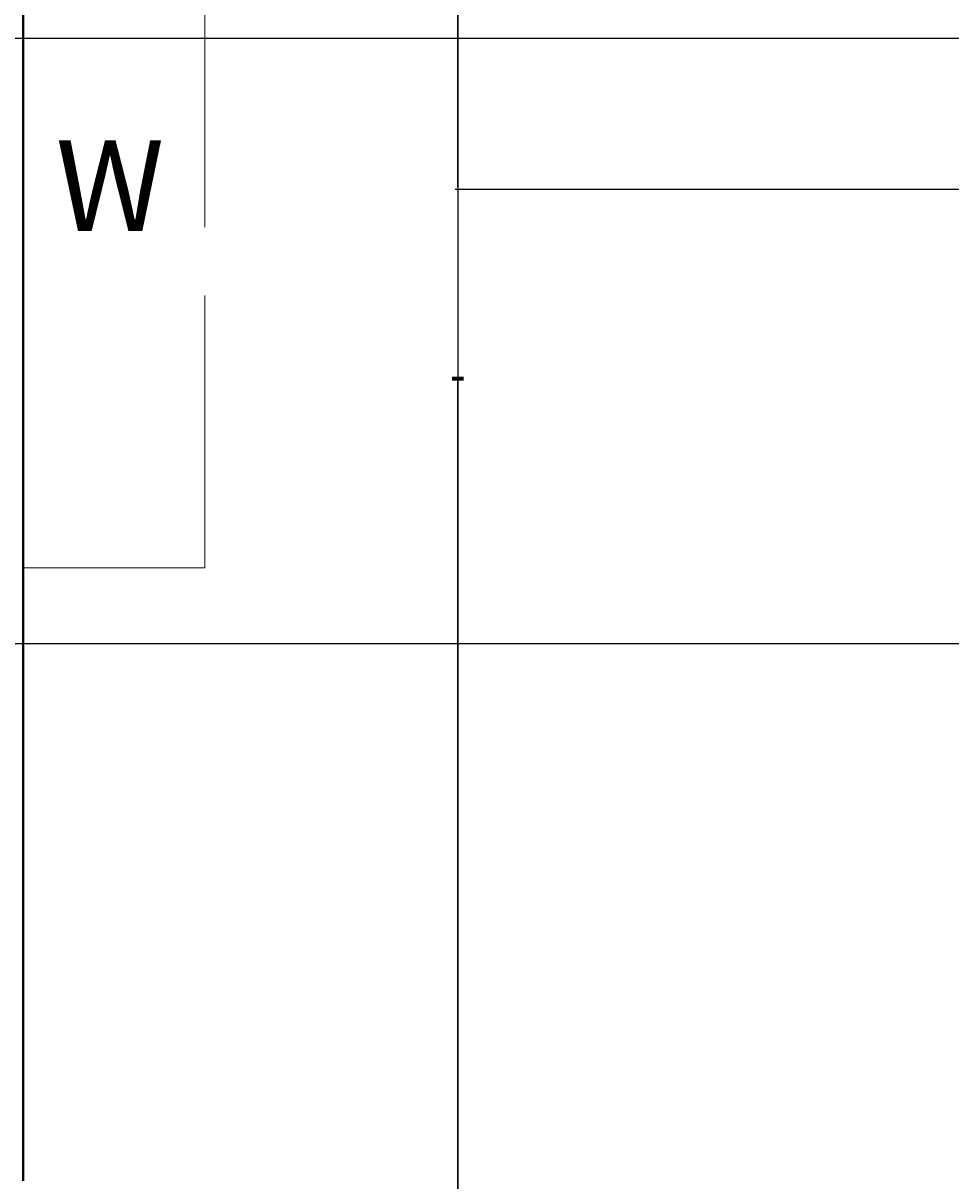
# Model space of a CAD drawing. Units: inches. Extents: x -301 to 715, y -607 to 364.
# Tile 103 of 141: x 133 to 194, y -10 to 67. Entities that reach past the tile are written whole.
import ezdxf

# ---------------------------------------------------------------- set-up
doc = ezdxf.new("R2010")
doc.units = ezdxf.units.IN
doc.header["$MEASUREMENT"] = 0
doc.linetypes.add('ACAD_ISO02W100', pattern=[15, 12, -3])
for name, color, linetype, lineweight in [('A-ANNO-DIMS', 2, 'Continuous', 18), ('A-ANNO-TEXT', 4, 'Continuous', 18), ('A-GLAZ-OVHD', 2, 'ACAD_ISO02W100', 18), ('A-WALL', 3, 'Continuous', 40)]:
    doc.layers.add(name, color=color, linetype=linetype, lineweight=lineweight)
doc.styles.get("Standard").update_dxf_attribs({"font": 'arial.ttf'})
doc.dimstyles.get("Standard").update_dxf_attribs({"dimtxt": 0.18, "dimasz": 0.18, "dimexe": 0.18, "dimexo": 0.0625, "dimgap": 0.09, "dimtad": 0, "dimtih": 1, "dimtoh": 1, "dimdec": 1, "dimzin": 0, "dimdsep": 46, "dimlunit": 4, "dimtxsty": 'Standard', "dimcen": 0.09, "dimclrd": 3, "dimclre": 4, "dimclrt": 6, "dimadec": 0, "dimazin": 0, "dimtfac": 1, "dimtdec": 1, "dimtofl": 0, "dimtmove": 0, "dimatfit": 3, "dimfxl": 1, "dimtfill": 2, "dimtfillclr": 51, "dimtolj": 1, "dimtzin": 0, "dimarcsym": 0})

# ---------------------------------------------------------------- blocks, each defined once
blk = doc.blocks.new('WIN-SHADE-50')
at = {"ltscale": 1.5}
for p, q in [((0, 0), (0, 12)), ((50, 12), (0, 12)), ((50, 0), (50, 12)), ((5, 0), (0, 0)), ((45, 0), (50, 0))]:
    blk.add_line(p, q, dxfattribs=at)
blk = doc.blocks.new('*D149')
at = {"layer": 'A-ANNO-DIMS', "color": 4, "lineweight": -2, "transparency": 16777216}
for p, q in [((-51.541, 65.682), (233.659, 65.682)), ((-51.541, 25.682), (233.659, 25.682))]:
    blk.add_line(p, q, dxfattribs=at)
at = {"layer": 'A-ANNO-DIMS', "color": 3, "lineweight": -2, "transparency": 16777216}
for p, q in [((233.479, 65.502), (233.479, 45.864)), ((233.479, 25.862), (233.479, 45.5))]:
    blk.add_line(p, q, dxfattribs=at)
at = {"layer": 'A-ANNO-DIMS', "color": 3, "transparency": 16777216}
for points in [[(233.449, 65.502), (233.509, 65.502), (233.479, 65.682)], [(233.449, 25.862), (233.509, 25.862), (233.479, 25.682)]]:
    blk.add_solid(points, dxfattribs=at)
at = {"layer": 'Defpoints', "color": 0, "transparency": 16777216}
for p in [(-51.603, 65.682), (-51.603, 25.682), (233.479, 25.682)]:
    blk.add_point(p, dxfattribs=at)
at = {"layer": 'A-ANNO-DIMS', "color": 6, "transparency": 16777216, "insert": (233.479, 45.682), "char_height": 0.18, "attachment_point": 5, "bg_fill": 1, "box_fill_scale": 1.25, "bg_fill_color": 51, "bg_fill_transparency": 0}
blk.add_mtext('\\A1;3\'-4"', dxfattribs=at)
blk = doc.blocks.new('*D162')
at = {"layer": 'A-ANNO-DIMS', "color": 4, "lineweight": -2, "transparency": 16777216}
for p, q in [((222.328, 320.182), (161.439, 320.182)), ((222.328, -233.818), (161.439, -233.818))]:
    blk.add_line(p, q, dxfattribs=at)
at = {"layer": 'A-ANNO-DIMS', "color": 3, "lineweight": -2, "transparency": 16777216}
for p, q in [((161.619, 320.002), (161.619, 43.364)), ((161.619, -233.638), (161.619, 43))]:
    blk.add_line(p, q, dxfattribs=at)
at = {"layer": 'A-ANNO-DIMS', "color": 3, "transparency": 16777216}
for points in [[(161.589, 320.002), (161.649, 320.002), (161.619, 320.182)], [(161.589, -233.638), (161.649, -233.638), (161.619, -233.818)]]:
    blk.add_solid(points, dxfattribs=at)
at = {"layer": 'Defpoints', "color": 0, "transparency": 16777216}
for p in [(161.619, 320.182), (222.39, 320.182), (222.39, -233.818)]:
    blk.add_point(p, dxfattribs=at)
at = {"layer": 'A-ANNO-DIMS', "color": 6, "transparency": 16777216, "insert": (161.619, 43.182), "char_height": 0.18, "attachment_point": 5, "bg_fill": 1, "box_fill_scale": 1.25, "bg_fill_color": 51, "bg_fill_transparency": 0}
blk.add_mtext('\\A1;46\'-2"', dxfattribs=at)
blk = doc.blocks.new('*D168')
at = {"layer": 'A-ANNO-DIMS', "color": 4, "lineweight": -2, "transparency": 16777216}
for p, q in [((222.328, 55.682), (161.439, 55.682)), ((222.328, -83.318), (161.439, -83.318))]:
    blk.add_line(p, q, dxfattribs=at)
at = {"layer": 'A-ANNO-DIMS', "color": 3, "lineweight": -2, "transparency": 16777216}
for p, q in [((161.619, 55.502), (161.619, -13.637)), ((161.619, -83.138), (161.619, -13.998))]:
    blk.add_line(p, q, dxfattribs=at)
at = {"layer": 'A-ANNO-DIMS', "color": 3, "transparency": 16777216}
for points in [[(161.589, 55.502), (161.649, 55.502), (161.619, 55.682)], [(161.589, -83.138), (161.649, -83.138), (161.619, -83.318)]]:
    blk.add_solid(points, dxfattribs=at)
at = {"layer": 'Defpoints', "color": 0, "transparency": 16777216}
for p in [(161.619, 55.682), (222.39, 55.682), (222.39, -83.318)]:
    blk.add_point(p, dxfattribs=at)
at = {"layer": 'A-ANNO-DIMS', "color": 6, "transparency": 16777216, "insert": (161.619, -13.818), "char_height": 0.18, "attachment_point": 5, "bg_fill": 1, "box_fill_scale": 1.25, "bg_fill_color": 51, "bg_fill_transparency": 0}
blk.add_mtext('\\A1;11\'-7"', dxfattribs=at)
blk = doc.blocks.new('*D169')
at = {"layer": 'A-ANNO-DIMS', "color": 4, "lineweight": -2, "transparency": 16777216}
for p, q in [((222.328, 183.182), (161.439, 183.182)), ((222.328, 55.682), (161.439, 55.682))]:
    blk.add_line(p, q, dxfattribs=at)
at = {"layer": 'A-ANNO-DIMS', "color": 3, "lineweight": -2, "transparency": 16777216}
for p, q in [((161.619, 183.002), (161.619, 119.615)), ((161.619, 55.862), (161.619, 119.249))]:
    blk.add_line(p, q, dxfattribs=at)
at = {"layer": 'A-ANNO-DIMS', "color": 3, "transparency": 16777216}
for points in [[(161.589, 183.002), (161.649, 183.002), (161.619, 183.182)], [(161.589, 55.862), (161.649, 55.862), (161.619, 55.682)]]:
    blk.add_solid(points, dxfattribs=at)
at = {"layer": 'Defpoints', "color": 0, "transparency": 16777216}
for p in [(161.619, 183.182), (222.39, 183.182), (222.39, 55.682)]:
    blk.add_point(p, dxfattribs=at)
at = {"layer": 'A-ANNO-DIMS', "color": 6, "transparency": 16777216, "insert": (161.619, 119.432), "char_height": 0.18, "attachment_point": 5, "bg_fill": 1, "box_fill_scale": 1.25, "bg_fill_color": 51, "bg_fill_transparency": 0}
blk.add_mtext('\\A1;10\'-7 1/2"', dxfattribs=at)

msp = doc.modelspace()

# ---------------------------------------------------------------- linework, layer by layer
at = {"layer": 'A-WALL'}
msp.add_line((132.897, -9.818), (132.897, 199.182), dxfattribs=at)

# ---------------------------------------------------------------- block references
at = {"layer": 'A-GLAZ-OVHD', "rotation": 270.0000000000001}
msp.add_blockref('WIN-SHADE-50', (132.896, 80.682), dxfattribs=at)

# ---------------------------------------------------------------- texts
at = {"layer": 'A-ANNO-TEXT'}
msp.add_text('W', height=6, dxfattribs=at).set_placement((135.041, 52.926))

# ---------------------------------------------------------------- dimensions: what is measured, and where the dimension line sits
at = {"layer": 'A-ANNO-DIMS'}
for base, p1, p2, picture, middle in [((161.619, 320.182), (222.39, -233.818), (222.39, 320.182), '*D162', (161.619, 43.182)), ((161.619, 183.182), (222.39, 55.682), (222.39, 183.182), '*D169', (161.619, 119.432)), ((233.479, 25.682), (-51.603, 65.682), (-51.603, 25.682), '*D149', (233.479, 45.682)), ((161.619, 55.682), (222.39, -83.318), (222.39, 55.682), '*D168', (161.619, -13.818))]:
    dim = msp.add_linear_dim(base=base, p1=p1, p2=p2, angle=90, dimstyle='Standard', override={"dimdec": 1, "dimlfac": 1, "dimrnd": 0, "dimzin": 1, "dimdsep": 46, "dimlunit": 4, "dimfrac": 2}, dxfattribs=at)
    dim.commit()
    dim.dimension.update_dxf_attribs({"geometry": picture, "text_midpoint": middle})

doc.saveas('drawing.dxf')
